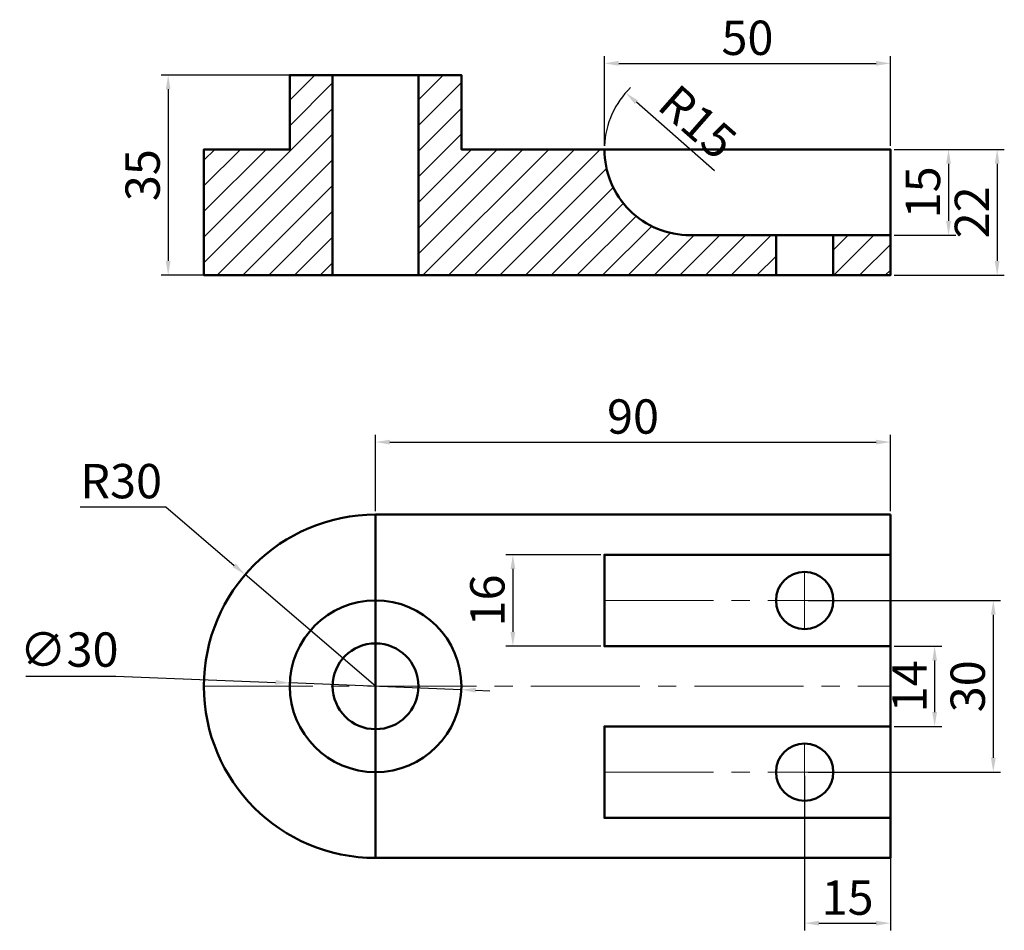
# Model space of a CAD drawing. Units: millimetres. Extents: x 7 to 179, y 8 to 167.
import ezdxf

# ---------------------------------------------------------------- set-up
doc = ezdxf.new("R2010")
doc.units = ezdxf.units.MM
doc.linetypes.add('CENTER2', pattern=[28.575, 19.05, -3.175, 3.175, -3.175])
for name, color, linetype, lineweight in [('M-CNTR', 1, 'CENTER2', 18), ('M-DIMS', 2, 'Continuous', 25), ('M-HATC', 8, 'Continuous', 18), ('M-OUTL', 7, 'Continuous', 50)]:
    doc.layers.add(name, color=color, linetype=linetype, lineweight=lineweight)
doc.styles.get("Standard").update_dxf_attribs({"font": 'arial.ttf'})
doc.dimstyles.new('ISO-25', dxfattribs={"dimtxt": 6, "dimasz": 2.5, "dimexe": 1.25, "dimexo": 0.625, "dimtad": 1, "dimtoh": 1, "dimdec": 0, "dimtxsty": 'Standard', "dimcen": 2.5, "dimadec": 0, "dimazin": 0, "dimtfac": 1, "dimtdec": 0, "dimtmove": 0, "dimatfit": 3, "dimfxl": 1, "dimarcsym": 0})

# ---------------------------------------------------------------- blocks, each defined once
blk = doc.blocks.new('*D1')
at = {"layer": 'Defpoints', "color": 0, "transparency": 16777216}
for p in [(69.33, 157.49), (33.08, 122.49), (69.33, 122.49)]:
    blk.add_point(p, dxfattribs=at)
at = {"layer": 'M-DIMS', "color": 0, "lineweight": -2, "transparency": 16777216}
for p, q in [((68.7, 157.49), (31.83, 157.49)), ((33.08, 154.99), (33.08, 124.99)), ((68.7, 122.49), (31.83, 122.49))]:
    blk.add_line(p, q, dxfattribs=at)
at = {"layer": 'M-DIMS', "color": 0, "transparency": 16777216}
for points in [[(32.66, 154.99), (33.5, 154.99), (33.08, 157.49)], [(32.66, 124.99), (33.5, 124.99), (33.08, 122.49)]]:
    blk.add_solid(points, dxfattribs=at)
at = {"layer": 'M-DIMS', "color": 0, "transparency": 16777216, "insert": (29.39, 139.99), "char_height": 6, "attachment_point": 5, "rotation": 90}
blk.add_mtext('35', dxfattribs=at)
blk = doc.blocks.new('*D2')
at = {"layer": 'Defpoints', "color": 0, "transparency": 16777216}
for p in [(113.05, 154.38), (124.33, 144.49)]:
    blk.add_point(p, dxfattribs=at)
at = {"layer": 'M-DIMS', "color": 0, "lineweight": -2, "transparency": 16777216}
blk.add_line((128.56, 140.77), (114.93, 152.73), dxfattribs=at)
blk.add_arc((124.33, 144.49), 15, 133.9724, 177.6127, dxfattribs=at)
at = {"layer": 'M-DIMS', "color": 0, "transparency": 16777216}
blk.add_solid([(115.2, 153.04), (114.65, 152.42), (113.05, 154.38)], dxfattribs=at)
at = {"layer": 'M-DIMS', "color": 0, "transparency": 16777216, "insert": (125.12, 148.7), "char_height": 6, "attachment_point": 5, "rotation": 318.7471}
blk.add_mtext('R15', dxfattribs=at)
blk = doc.blocks.new('*D3')
at = {"layer": 'Defpoints', "color": 0, "transparency": 16777216}
for p in [(159.33, 159.53), (109.33, 144.49), (159.33, 144.49)]:
    blk.add_point(p, dxfattribs=at)
at = {"layer": 'M-DIMS', "color": 0, "lineweight": -2, "transparency": 16777216}
for p, q in [((109.33, 145.11), (109.33, 160.78)), ((159.33, 145.11), (159.33, 160.78)), ((111.83, 159.53), (156.83, 159.53))]:
    blk.add_line(p, q, dxfattribs=at)
at = {"layer": 'M-DIMS', "color": 0, "transparency": 16777216}
for points in [[(111.83, 159.95), (111.83, 159.12), (109.33, 159.53)], [(156.83, 159.95), (156.83, 159.12), (159.33, 159.53)]]:
    blk.add_solid(points, dxfattribs=at)
at = {"layer": 'M-DIMS', "color": 0, "transparency": 16777216, "insert": (134.33, 163.22), "char_height": 6, "attachment_point": 5}
blk.add_mtext('50', dxfattribs=at)
blk = doc.blocks.new('*D4')
at = {"layer": 'Defpoints', "color": 0, "transparency": 16777216}
for p in [(159.33, 144.49), (159.33, 129.49), (169.48, 129.49)]:
    blk.add_point(p, dxfattribs=at)
at = {"layer": 'M-DIMS', "color": 0, "lineweight": -2, "transparency": 16777216}
for p, q in [((159.95, 144.49), (170.73, 144.49)), ((169.48, 141.99), (169.48, 131.99)), ((159.95, 129.49), (170.73, 129.49))]:
    blk.add_line(p, q, dxfattribs=at)
at = {"layer": 'M-DIMS', "color": 0, "transparency": 16777216}
for points in [[(169.06, 141.99), (169.9, 141.99), (169.48, 144.49)], [(169.06, 131.99), (169.9, 131.99), (169.48, 129.49)]]:
    blk.add_solid(points, dxfattribs=at)
at = {"layer": 'M-DIMS', "color": 0, "transparency": 16777216, "insert": (165.79, 136.99), "char_height": 6, "attachment_point": 5, "rotation": 90}
blk.add_mtext('15', dxfattribs=at)
blk = doc.blocks.new('*D5')
at = {"layer": 'Defpoints', "color": 0, "transparency": 16777216}
for p in [(159.33, 144.49), (159.33, 122.49), (177.98, 122.49)]:
    blk.add_point(p, dxfattribs=at)
at = {"layer": 'M-DIMS', "color": 0, "lineweight": -2, "transparency": 16777216}
for p, q in [((159.95, 144.49), (179.23, 144.49)), ((177.98, 141.99), (177.98, 124.99)), ((159.95, 122.49), (179.23, 122.49))]:
    blk.add_line(p, q, dxfattribs=at)
at = {"layer": 'M-DIMS', "color": 0, "transparency": 16777216}
for points in [[(177.56, 141.99), (178.39, 141.99), (177.98, 144.49)], [(177.56, 124.99), (178.39, 124.99), (177.98, 122.49)]]:
    blk.add_solid(points, dxfattribs=at)
at = {"layer": 'M-DIMS', "color": 0, "transparency": 16777216, "insert": (174.34, 133.49), "char_height": 6, "attachment_point": 5, "rotation": 90}
blk.add_mtext('22', dxfattribs=at)
blk = doc.blocks.new('*D6')
at = {"layer": 'Defpoints', "color": 0, "transparency": 16777216}
for p in [(159.33, 93.34), (69.33, 80.66), (159.33, 80.66)]:
    blk.add_point(p, dxfattribs=at)
at = {"layer": 'M-DIMS', "color": 0, "lineweight": -2, "transparency": 16777216}
for p, q in [((69.33, 81.29), (69.33, 94.59)), ((71.83, 93.34), (156.83, 93.34)), ((159.33, 81.29), (159.33, 94.59))]:
    blk.add_line(p, q, dxfattribs=at)
at = {"layer": 'M-DIMS', "color": 0, "transparency": 16777216}
for points in [[(71.83, 93.75), (71.83, 92.92), (69.33, 93.34)], [(156.83, 93.75), (156.83, 92.92), (159.33, 93.34)]]:
    blk.add_solid(points, dxfattribs=at)
at = {"layer": 'M-DIMS', "color": 0, "transparency": 16777216, "insert": (114.33, 97.03), "char_height": 6, "attachment_point": 5}
blk.add_mtext('90', dxfattribs=at)
blk = doc.blocks.new('*D7')
at = {"layer": 'Defpoints', "color": 0, "transparency": 16777216}
for p in [(46.54, 70.17), (69.33, 50.66)]:
    blk.add_point(p, dxfattribs=at)
at = {"layer": 'M-DIMS', "color": 0, "lineweight": -2, "transparency": 16777216}
for p, q in [((17.71, 82.05), (32.66, 82.05)), ((32.66, 82.05), (44.64, 71.8)), ((69.33, 50.66), (46.54, 70.17))]:
    blk.add_line(p, q, dxfattribs=at)
at = {"layer": 'M-DIMS', "color": 0, "transparency": 16777216}
blk.add_solid([(44.91, 72.11), (44.37, 71.48), (46.54, 70.17)], dxfattribs=at)
at = {"layer": 'M-DIMS', "color": 0, "transparency": 16777216, "insert": (24.87, 85.74), "char_height": 6, "attachment_point": 5}
blk.add_mtext('R30', dxfattribs=at)
blk = doc.blocks.new('*D8')
at = {"layer": 'Defpoints', "color": 0, "transparency": 16777216}
for p in [(54.34, 51.25), (84.31, 50.07)]:
    blk.add_point(p, dxfattribs=at)
at = {"layer": 'M-DIMS', "color": 0, "lineweight": -2, "transparency": 16777216}
for p, q in [((8.21, 52.45), (23.94, 52.45)), ((23.94, 52.45), (51.84, 51.35)), ((84.31, 50.07), (54.34, 51.25)), ((86.81, 49.97), (89.31, 49.87))]:
    blk.add_line(p, q, dxfattribs=at)
at = {"layer": 'M-DIMS', "color": 0, "transparency": 16777216}
for points in [[(51.86, 51.77), (51.82, 50.93), (54.34, 51.25)], [(86.83, 50.39), (86.8, 49.56), (84.31, 50.07)]]:
    blk.add_solid(points, dxfattribs=at)
at = {"layer": 'M-DIMS', "color": 0, "transparency": 16777216, "insert": (15.77, 56.3), "char_height": 6, "attachment_point": 5}
blk.add_mtext('∅30', dxfattribs=at)
blk = doc.blocks.new('*D9')
at = {"layer": 'Defpoints', "color": 0, "transparency": 16777216}
for p in [(144.33, 35.66), (159.33, 35.66), (159.33, 9.26)]:
    blk.add_point(p, dxfattribs=at)
at = {"layer": 'M-DIMS', "color": 0, "lineweight": -2, "transparency": 16777216}
for p, q in [((144.33, 35.04), (144.33, 8.01)), ((159.33, 35.04), (159.33, 8.01)), ((146.83, 9.26), (156.83, 9.26))]:
    blk.add_line(p, q, dxfattribs=at)
at = {"layer": 'M-DIMS', "color": 0, "transparency": 16777216}
for points in [[(146.83, 9.68), (146.83, 8.85), (144.33, 9.26)], [(156.83, 9.68), (156.83, 8.85), (159.33, 9.26)]]:
    blk.add_solid(points, dxfattribs=at)
at = {"layer": 'M-DIMS', "color": 0, "transparency": 16777216, "insert": (151.83, 12.95), "char_height": 6, "attachment_point": 5}
blk.add_mtext('15', dxfattribs=at)
blk = doc.blocks.new('*D10')
at = {"layer": 'Defpoints', "color": 0, "transparency": 16777216}
for p in [(159.33, 57.66), (159.33, 43.66), (167.05, 43.66)]:
    blk.add_point(p, dxfattribs=at)
at = {"layer": 'M-DIMS', "color": 0, "lineweight": -2, "transparency": 16777216}
for p, q in [((159.95, 57.66), (168.3, 57.66)), ((167.05, 55.16), (167.05, 46.16)), ((159.95, 43.66), (168.3, 43.66))]:
    blk.add_line(p, q, dxfattribs=at)
at = {"layer": 'M-DIMS', "color": 0, "transparency": 16777216}
for points in [[(166.64, 55.16), (167.47, 55.16), (167.05, 57.66)], [(166.64, 46.16), (167.47, 46.16), (167.05, 43.66)]]:
    blk.add_solid(points, dxfattribs=at)
at = {"layer": 'M-DIMS', "color": 0, "transparency": 16777216, "insert": (163.41, 50.66), "char_height": 6, "attachment_point": 5, "rotation": 90}
blk.add_mtext('14', dxfattribs=at)
blk = doc.blocks.new('*D11')
at = {"layer": 'Defpoints', "color": 0, "transparency": 16777216}
for p in [(144.33, 65.66), (144.33, 35.66), (177.3, 35.66)]:
    blk.add_point(p, dxfattribs=at)
at = {"layer": 'M-DIMS', "color": 0, "lineweight": -2, "transparency": 16777216}
for p, q in [((144.95, 65.66), (178.55, 65.66)), ((177.3, 63.16), (177.3, 38.16)), ((144.95, 35.66), (178.55, 35.66))]:
    blk.add_line(p, q, dxfattribs=at)
at = {"layer": 'M-DIMS', "color": 0, "transparency": 16777216}
for points in [[(176.89, 63.16), (177.72, 63.16), (177.3, 65.66)], [(176.89, 38.16), (177.72, 38.16), (177.3, 35.66)]]:
    blk.add_solid(points, dxfattribs=at)
at = {"layer": 'M-DIMS', "color": 0, "transparency": 16777216, "insert": (173.61, 50.66), "char_height": 6, "attachment_point": 5, "rotation": 90}
blk.add_mtext('30', dxfattribs=at)
blk = doc.blocks.new('*D12')
at = {"layer": 'Defpoints', "color": 0, "transparency": 16777216}
for p in [(109.33, 73.66), (93.33, 57.66), (109.33, 57.66)]:
    blk.add_point(p, dxfattribs=at)
at = {"layer": 'M-DIMS', "color": 0, "lineweight": -2, "transparency": 16777216}
for p, q in [((108.7, 73.66), (92.08, 73.66)), ((93.33, 71.16), (93.33, 60.16)), ((108.7, 57.66), (92.08, 57.66))]:
    blk.add_line(p, q, dxfattribs=at)
at = {"layer": 'M-DIMS', "color": 0, "transparency": 16777216}
for points in [[(92.92, 71.16), (93.75, 71.16), (93.33, 73.66)], [(92.92, 60.16), (93.75, 60.16), (93.33, 57.66)]]:
    blk.add_solid(points, dxfattribs=at)
at = {"layer": 'M-DIMS', "color": 0, "transparency": 16777216, "insert": (89.65, 65.66), "char_height": 6, "attachment_point": 5, "rotation": 90}
blk.add_mtext('16', dxfattribs=at)

msp = doc.modelspace()

# ---------------------------------------------------------------- hatches: boundary and pattern name
at = {"layer": 'M-HATC'}
h = msp.add_hatch(dxfattribs=at)
h.set_pattern_fill('ANSI31', color=256)
h.paths.add_polyline_path([(61.83, 157.49), (54.33, 157.49), (54.33, 144.49), (39.33, 144.49), (39.33, 122.49), (61.83, 122.49)])
h.paths.add_polyline_path([(109.33, 144.49), (84.33, 144.49), (84.33, 157.49), (76.83, 157.49), (76.83, 122.49), (139.33, 122.49), (139.33, 129.49), (124.33, 129.49, -0.414214)])
h.paths.add_polyline_path([(159.33, 129.49), (149.33, 129.49), (149.33, 122.49), (159.33, 122.49)])

# ---------------------------------------------------------------- linework, layer by layer
at = {"layer": 'M-CNTR'}
for p, q in [((144.33, 60.66), (144.33, 70.66)), ((109.33, 65.66), (159.33, 65.66)), ((39.33, 50.66), (159.33, 50.66)), ((144.33, 30.66), (144.33, 40.66)), ((109.33, 35.66), (159.33, 35.66))]:
    msp.add_line(p, q, dxfattribs=at)
at = {"layer": 'M-OUTL'}
for p, q in [((61.83, 122.49), (61.83, 157.49)), ((76.83, 122.49), (76.83, 157.49)), ((139.33, 122.49), (139.33, 129.49)), ((149.33, 122.49), (149.33, 129.49)), ((69.33, 80.66), (159.33, 80.66)), ((159.33, 80.66), (159.33, 20.66)), ((69.33, 20.66), (159.33, 20.66))]:
    msp.add_line(p, q, dxfattribs=at)
for points in [[(109.33, 144.49), (109.33, 144.49), (84.33, 144.49), (84.33, 157.49), (54.33, 157.49), (54.33, 144.49), (39.33, 144.49), (39.33, 122.49), (159.33, 122.49), (159.33, 129.49)], [(159.33, 73.66), (109.33, 73.66), (109.33, 57.66), (159.33, 57.66)], [(159.33, 27.66), (109.33, 27.66), (109.33, 43.66), (159.33, 43.66)]]:
    msp.add_lwpolyline(points, dxfattribs=at)
for points in [[(109.33, 144.49), (159.33, 144.49), (159.33, 129.49), (124.33, 129.49, -0.414214)], [(69.33, 80.66, 1), (69.33, 20.66)]]:
    msp.add_lwpolyline(points, format="xyb", close=True, dxfattribs=at)
for centre, radius in [((144.33, 65.66), 5), ((69.33, 50.66), 15), ((69.33, 50.66), 7.5), ((144.33, 35.66), 5)]:
    msp.add_circle(centre, radius, dxfattribs=at)

# ---------------------------------------------------------------- dimensions: what is measured, and where the dimension line sits
at = {"layer": 'M-DIMS'}
for base, p1, p2, picture, middle in [((159.33, 159.53), (109.33, 144.49), (159.33, 144.49), '*D3', (134.33, 163.22)), ((159.33, 93.34), (69.33, 80.66), (159.33, 80.66), '*D6', (114.33, 97.03)), ((159.33, 9.26), (144.33, 35.66), (159.33, 35.66), '*D9', (151.83, 12.95))]:
    dim = msp.add_linear_dim(base=base, p1=p1, p2=p2, dimstyle='ISO-25', override={"dimclrd": 0, "dimclre": 0, "dimclrt": 0}, dxfattribs=at)
    dim.commit()
    dim.dimension.update_dxf_attribs({"geometry": picture, "text_midpoint": middle})
for base, p1, p2, picture, middle in [((33.08, 122.49), (69.33, 157.49), (69.33, 122.49), '*D1', (29.39, 139.99)), ((169.48, 129.49), (159.33, 144.49), (159.33, 129.49), '*D4', (165.79, 136.99)), ((177.98, 122.49), (159.33, 144.49), (159.33, 122.49), '*D5', (174.34, 133.49)), ((93.33, 57.66), (109.33, 73.66), (109.33, 57.66), '*D12', (89.65, 65.66)), ((177.3, 35.66), (144.33, 65.66), (144.33, 35.66), '*D11', (173.61, 50.66)), ((167.05, 43.66), (159.33, 57.66), (159.33, 43.66), '*D10', (163.41, 50.66))]:
    dim = msp.add_linear_dim(base=base, p1=p1, p2=p2, angle=90, dimstyle='ISO-25', override={"dimclrd": 0, "dimclre": 0, "dimclrt": 0}, dxfattribs=at)
    dim.commit()
    dim.dimension.update_dxf_attribs({"geometry": picture, "text_midpoint": middle})
for center, mpoint, picture, middle in [((124.33, 144.49), (113.05, 154.38), '*D2', (122.68, 145.93)), ((69.33, 50.66), (46.54, 70.17), '*D7', (24.87, 82.05))]:
    dim = msp.add_radius_dim(center=center, mpoint=mpoint, dimstyle='ISO-25', override={"dimclrd": 0, "dimclre": 0, "dimclrt": 0}, dxfattribs=at)
    dim.commit()
    dim.dimension.update_dxf_attribs({"geometry": picture, "text_midpoint": middle, "dimtype": 164})
dim = msp.add_diameter_dim_2p(p1=(84.31, 50.07), p2=(54.34, 51.25), dimstyle='ISO-25', override={"dimclrd": 0, "dimclre": 0, "dimclrt": 0}, dxfattribs=at)
dim.commit()
dim.dimension.update_dxf_attribs({"geometry": '*D8', "text_midpoint": (23.94, 52.45), "dimtype": 163})

doc.saveas('drawing.dxf')
